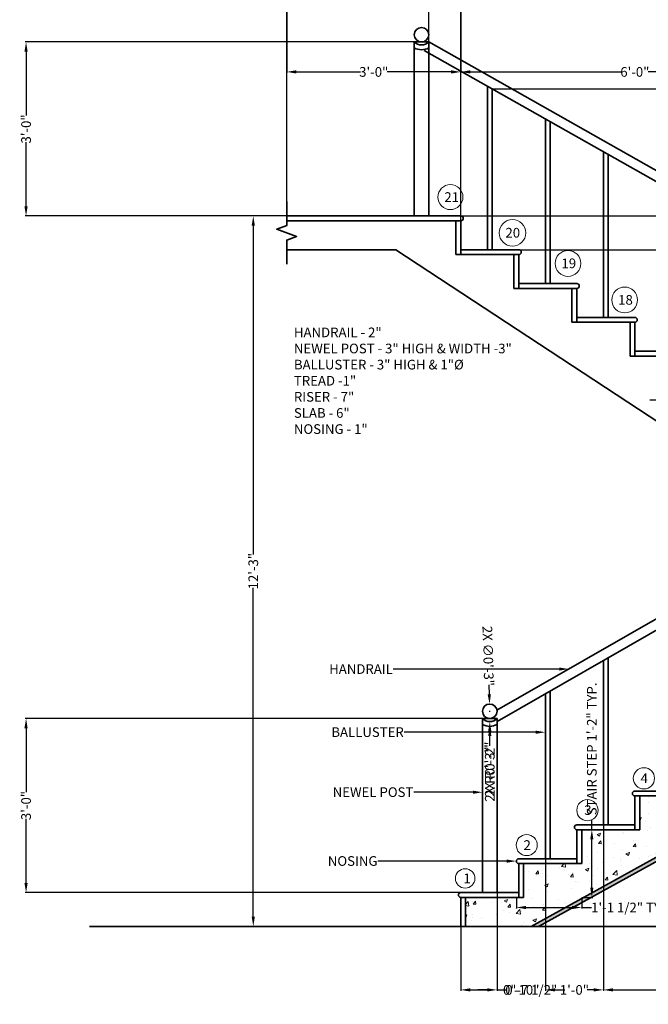
# Model space of a CAD drawing. Units: inches. Extents: x 865 to 1137, y 672 to 989.
# Tile 1 of 3: x 865 to 995, y 672 to 876. Entities that reach past the tile are written whole.
import ezdxf
from ezdxf import colors
from ezdxf.entities.mleader import LeaderData, LeaderLine
from ezdxf.math import Vec2, Vec3

# ---------------------------------------------------------------- set-up
doc = ezdxf.new("R2010")
doc.units = ezdxf.units.IN
doc.header["$LTSCALE"] = 0.1
doc.header["$MEASUREMENT"] = 0
for name, color, linetype, lineweight in [('A-ANNO-DIMS', 2, 'Continuous', 18), ('A-ANNO-SYMB', 3, 'Continuous', 18), ('A-ANNO-TEXT', 3, 'Continuous', 18), ('A-SECT', 7, 'Continuous', 35), ('A-SECT-PATT', 8, 'Continuous', 13)]:
    doc.layers.add(name, color=color, linetype=linetype, lineweight=lineweight)
doc.styles.get("Standard").update_dxf_attribs({"font": 'arial.ttf', "height": 2})
doc.dimstyles.get("Standard").update_dxf_attribs({"dimtxt": 2, "dimasz": 2, "dimexe": 0.18, "dimexo": 0.0625, "dimgap": 0.09, "dimtad": 0, "dimdec": 0, "dimzin": 0, "dimdsep": 46, "dimlunit": 3, "dimtxsty": 'Standard', "dimcen": 0.09, "dimadec": 0, "dimazin": 0, "dimtfac": 1, "dimtdec": 0, "dimtofl": 0, "dimtmove": 0, "dimatfit": 3, "dimfxl": 1, "dimtolj": 1, "dimtzin": 0, "dimarcsym": 0})

# ---------------------------------------------------------------- blocks, each defined once
blk = doc.blocks.new('*D6')
at = {"layer": 'A-ANNO-DIMS', "color": 0, "lineweight": -2, "transparency": 16777216}
for p, q in [((920.3, 835.55), (913.27, 835.55)), ((913.45, 833.55), (913.45, 765.48)), ((913.45, 690.55), (913.45, 758.62)), ((920.3, 688.55), (913.27, 688.55))]:
    blk.add_line(p, q, dxfattribs=at)
at = {"layer": 'A-ANNO-DIMS', "color": 0, "transparency": 16777216}
for points in [[(913.11, 833.55), (913.78, 833.55), (913.45, 835.55)], [(913.11, 690.55), (913.78, 690.55), (913.45, 688.55)]]:
    blk.add_solid(points, dxfattribs=at)
at = {"layer": 'Defpoints', "color": 0, "transparency": 16777216}
for p in [(920.36, 835.55), (913.45, 688.55), (920.36, 688.55)]:
    blk.add_point(p, dxfattribs=at)
at = {"layer": 'A-ANNO-DIMS', "color": 0, "transparency": 16777216, "insert": (913.45, 762.05), "char_height": 2, "attachment_point": 5, "rotation": 90}
blk.add_mtext('\\A1;12\'-3"', dxfattribs=at)
blk = doc.blocks.new('STAIR-STEP-SECT')
for p, q in [((13.5, 7), (13.5, 14)), ((0.5, 8), (12.5, 8)), ((0.5, 0), (0.5, 7)), ((0.5, 7), (13.5, 7))]:
    blk.add_line(p, q)
blk.add_arc((0.5, 7.5), 0.5, 90, 270)
blk = doc.blocks.new('*D9')
at = {"layer": 'A-ANNO-DIMS', "color": 0, "lineweight": -2, "transparency": 16777216}
for p, q in [((983.46, 708.55), (983.46, 710.55)), ((981.42, 708.55), (983.64, 708.55)), ((983.46, 696.55), (983.46, 706.55)), ((981.42, 694.55), (983.64, 694.55))]:
    blk.add_line(p, q, dxfattribs=at)
at = {"layer": 'A-ANNO-DIMS', "color": 0, "transparency": 16777216}
for points in [[(983.13, 706.55), (983.79, 706.55), (983.46, 708.55)], [(983.13, 696.55), (983.79, 696.55), (983.46, 694.55)]]:
    blk.add_solid(points, dxfattribs=at)
at = {"layer": 'Defpoints', "color": 0, "transparency": 16777216}
for p in [(981.36, 708.55), (983.46, 708.55), (981.36, 694.55)]:
    blk.add_point(p, dxfattribs=at)
at = {"layer": 'A-ANNO-DIMS', "color": 0, "transparency": 16777216, "insert": (983.46, 725.27), "char_height": 2, "attachment_point": 5, "rotation": 90}
blk.add_mtext('\\A1;STAIR STEP 1\'-2" TYP.', dxfattribs=at)
blk = doc.blocks.new('*D10')
at = {"layer": 'A-ANNO-DIMS', "color": 0, "lineweight": -2, "transparency": 16777216}
for p, q in [((967.86, 694.49), (967.86, 692.27)), ((981.36, 694.49), (981.36, 692.27)), ((969.86, 692.45), (979.36, 692.45)), ((981.36, 692.45), (983.36, 692.45))]:
    blk.add_line(p, q, dxfattribs=at)
at = {"layer": 'A-ANNO-DIMS', "color": 0, "transparency": 16777216}
for points in [[(969.86, 692.79), (969.86, 692.12), (967.86, 692.45)], [(979.36, 692.79), (979.36, 692.12), (981.36, 692.45)]]:
    blk.add_solid(points, dxfattribs=at)
at = {"layer": 'Defpoints', "color": 0, "transparency": 16777216}
for p in [(967.86, 694.55), (981.36, 694.55), (981.36, 692.45)]:
    blk.add_point(p, dxfattribs=at)
at = {"layer": 'A-ANNO-DIMS', "color": 0, "transparency": 16777216, "insert": (991.78, 692.45), "char_height": 2, "attachment_point": 5}
blk.add_mtext('\\A1;1\'-1 1/2" TYP.', dxfattribs=at)
blk = doc.blocks.new('*D12')
at = {"layer": 'A-ANNO-DIMS', "color": 0, "lineweight": -2, "transparency": 16777216}
for p, q in [((956.36, 891.19), (956.36, 865.17)), ((920.36, 880.69), (920.36, 865.17)), ((922.36, 865.35), (935.61, 865.35)), ((954.36, 865.35), (941.11, 865.35))]:
    blk.add_line(p, q, dxfattribs=at)
at = {"layer": 'A-ANNO-DIMS', "color": 0, "transparency": 16777216}
for points in [[(922.36, 865.69), (922.36, 865.02), (920.36, 865.35)], [(954.36, 865.69), (954.36, 865.02), (956.36, 865.35)]]:
    blk.add_solid(points, dxfattribs=at)
at = {"layer": 'Defpoints', "color": 0, "transparency": 16777216}
for p in [(956.36, 891.25), (920.36, 880.75), (956.36, 865.35)]:
    blk.add_point(p, dxfattribs=at)
at = {"layer": 'A-ANNO-DIMS', "color": 0, "transparency": 16777216, "insert": (938.36, 865.35), "char_height": 2, "attachment_point": 5}
blk.add_mtext('\\A1;3\'-0"', dxfattribs=at)
blk = doc.blocks.new('*D13')
at = {"layer": 'A-ANNO-DIMS', "color": 0, "lineweight": -2, "transparency": 16777216}
for p, q in [((956.36, 891.19), (956.36, 865.17)), ((1028.36, 880.69), (1028.36, 865.17)), ((958.36, 865.35), (989.6, 865.35)), ((1026.36, 865.35), (995.11, 865.35))]:
    blk.add_line(p, q, dxfattribs=at)
at = {"layer": 'A-ANNO-DIMS', "color": 0, "transparency": 16777216}
for points in [[(958.36, 865.69), (958.36, 865.02), (956.36, 865.35)], [(1026.36, 865.69), (1026.36, 865.02), (1028.36, 865.35)]]:
    blk.add_solid(points, dxfattribs=at)
at = {"layer": 'Defpoints', "color": 0, "transparency": 16777216}
for p in [(956.36, 891.25), (1028.36, 880.75), (1028.36, 865.35)]:
    blk.add_point(p, dxfattribs=at)
at = {"layer": 'A-ANNO-DIMS', "color": 0, "transparency": 16777216, "insert": (992.36, 865.35), "char_height": 2, "attachment_point": 5}
blk.add_mtext('\\A1;6\'-0"', dxfattribs=at)
blk = doc.blocks.new('*D21')
at = {"layer": 'A-ANNO-DIMS', "color": 0, "lineweight": -2, "transparency": 16777216}
for p, q in [((920.36, 835.61), (920.36, 887.89)), ((922.36, 887.71), (994.85, 887.71)), ((1078.86, 887.71), (1006.37, 887.71)), ((1080.86, 861.4), (1080.86, 887.89))]:
    blk.add_line(p, q, dxfattribs=at)
at = {"layer": 'A-ANNO-DIMS', "color": 0, "transparency": 16777216}
for points in [[(922.36, 888.04), (922.36, 887.37), (920.36, 887.71)], [(1078.86, 888.04), (1078.86, 887.37), (1080.86, 887.71)]]:
    blk.add_solid(points, dxfattribs=at)
at = {"layer": 'Defpoints', "color": 0, "transparency": 16777216}
for p in [(1080.86, 887.71), (1080.86, 861.34), (920.36, 835.55)]:
    blk.add_point(p, dxfattribs=at)
at = {"layer": 'A-ANNO-DIMS', "color": 0, "transparency": 16777216, "insert": (1000.61, 887.71), "char_height": 2, "attachment_point": 5}
blk.add_mtext('\\A1;13\'-4 1/2"', dxfattribs=at)
blk = doc.blocks.new('*D22')
at = {"layer": 'A-ANNO-DIMS', "color": 0, "lineweight": -2, "transparency": 16777216}
for p, q in [((985.86, 709.49), (985.86, 675.22)), ((1070.36, 688.49), (1070.36, 675.22)), ((987.86, 675.4), (1023.04, 675.4)), ((1068.36, 675.4), (1033.18, 675.4))]:
    blk.add_line(p, q, dxfattribs=at)
at = {"layer": 'A-ANNO-DIMS', "color": 0, "transparency": 16777216}
for points in [[(987.86, 675.74), (987.86, 675.07), (985.86, 675.4)], [(1068.36, 675.74), (1068.36, 675.07), (1070.36, 675.4)]]:
    blk.add_solid(points, dxfattribs=at)
at = {"layer": 'Defpoints', "color": 0, "transparency": 16777216}
for p in [(985.86, 709.55), (1070.36, 688.55), (1070.36, 675.4)]:
    blk.add_point(p, dxfattribs=at)
at = {"layer": 'A-ANNO-DIMS', "color": 0, "transparency": 16777216, "insert": (1028.11, 675.4), "char_height": 2, "attachment_point": 5}
blk.add_mtext('\\A1;7\'-0 1/2"', dxfattribs=at)
blk = doc.blocks.new('*D23')
at = {"layer": 'A-ANNO-DIMS', "color": 0, "lineweight": -2, "transparency": 16777216}
for p, q in [((960.8, 731.55), (866.28, 731.55)), ((866.46, 729.55), (866.46, 716.3)), ((866.46, 697.55), (866.46, 710.8)), ((960.8, 695.55), (866.28, 695.55))]:
    blk.add_line(p, q, dxfattribs=at)
at = {"layer": 'A-ANNO-DIMS', "color": 0, "transparency": 16777216}
for points in [[(866.12, 729.55), (866.79, 729.55), (866.46, 731.55)], [(866.12, 697.55), (866.79, 697.55), (866.46, 695.55)]]:
    blk.add_solid(points, dxfattribs=at)
at = {"layer": 'Defpoints', "color": 0, "transparency": 16777216}
for p in [(866.46, 731.55), (960.86, 731.55), (960.86, 695.55)]:
    blk.add_point(p, dxfattribs=at)
at = {"layer": 'A-ANNO-DIMS', "color": 0, "transparency": 16777216, "insert": (866.46, 713.55), "char_height": 2, "attachment_point": 5, "rotation": 90}
blk.add_mtext('\\A1;3\'-0"', dxfattribs=at)
blk = doc.blocks.new('*D24')
at = {"layer": 'A-ANNO-DIMS', "color": 0, "lineweight": -2, "transparency": 16777216}
for p, q in [((963.86, 695.49), (963.86, 675.22)), ((956.36, 688.49), (956.36, 675.22)), ((958.36, 675.4), (961.86, 675.4)), ((963.86, 675.4), (965.86, 675.4))]:
    blk.add_line(p, q, dxfattribs=at)
at = {"layer": 'A-ANNO-DIMS', "color": 0, "transparency": 16777216}
for points in [[(958.36, 675.74), (958.36, 675.07), (956.36, 675.4)], [(961.86, 675.74), (961.86, 675.07), (963.86, 675.4)]]:
    blk.add_solid(points, dxfattribs=at)
at = {"layer": 'Defpoints', "color": 0, "transparency": 16777216}
for p in [(963.86, 695.55), (956.36, 688.55), (963.86, 675.4)]:
    blk.add_point(p, dxfattribs=at)
at = {"layer": 'A-ANNO-DIMS', "color": 0, "transparency": 16777216, "insert": (970.94, 675.4), "char_height": 2, "attachment_point": 5}
blk.add_mtext('\\A1;0\'-7 1/2"', dxfattribs=at)
blk = doc.blocks.new('*D25')
at = {"layer": 'A-ANNO-DIMS', "color": 0, "lineweight": -2, "transparency": 16777216}
for p, q in [((962.92, 861.84), (1124.29, 861.84)), ((1124.11, 859.84), (1124.11, 850.29)), ((1124.11, 830.55), (1124.11, 840.1)), ((962.92, 828.55), (1124.29, 828.55))]:
    blk.add_line(p, q, dxfattribs=at)
at = {"layer": 'A-ANNO-DIMS', "color": 0, "transparency": 16777216}
for points in [[(1123.78, 859.84), (1124.44, 859.84), (1124.11, 861.84)], [(1123.78, 830.55), (1124.44, 830.55), (1124.11, 828.55)]]:
    blk.add_solid(points, dxfattribs=at)
at = {"layer": 'Defpoints', "color": 0, "transparency": 16777216}
for p in [(962.86, 861.84), (1124.11, 861.84), (962.86, 828.55)]:
    blk.add_point(p, dxfattribs=at)
at = {"layer": 'A-ANNO-DIMS', "color": 0, "transparency": 16777216, "insert": (1124.11, 845.19), "char_height": 2, "attachment_point": 5, "rotation": 90}
blk.add_mtext('\\A1;2\'-9 1/2"', dxfattribs=at)
blk = doc.blocks.new('*D26')
at = {"layer": 'A-ANNO-DIMS', "color": 0, "lineweight": -2, "transparency": 16777216}
for p, q in [((973.86, 702.49), (973.86, 675.22)), ((963.86, 695.49), (963.86, 675.22)), ((961.86, 675.4), (959.86, 675.4)), ((975.86, 675.4), (977.86, 675.4))]:
    blk.add_line(p, q, dxfattribs=at)
at = {"layer": 'A-ANNO-DIMS', "color": 0, "transparency": 16777216}
for points in [[(961.86, 675.74), (961.86, 675.07), (963.86, 675.4)], [(975.86, 675.74), (975.86, 675.07), (973.86, 675.4)]]:
    blk.add_solid(points, dxfattribs=at)
at = {"layer": 'Defpoints', "color": 0, "transparency": 16777216}
for p in [(973.86, 702.55), (963.86, 695.55), (973.86, 675.4)]:
    blk.add_point(p, dxfattribs=at)
at = {"layer": 'A-ANNO-DIMS', "color": 0, "transparency": 16777216, "insert": (968.86, 675.4), "char_height": 2, "attachment_point": 5}
blk.add_mtext('\\A1;0\'-10"', dxfattribs=at)
blk = doc.blocks.new('*D27')
at = {"layer": 'A-ANNO-DIMS', "color": 0, "lineweight": -2, "transparency": 16777216}
for p, q in [((985.86, 709.49), (985.86, 675.22)), ((973.86, 702.49), (973.86, 675.22)), ((975.86, 675.4), (977.2, 675.4)), ((983.86, 675.4), (982.51, 675.4))]:
    blk.add_line(p, q, dxfattribs=at)
at = {"layer": 'A-ANNO-DIMS', "color": 0, "transparency": 16777216}
for points in [[(975.86, 675.74), (975.86, 675.07), (973.86, 675.4)], [(983.86, 675.74), (983.86, 675.07), (985.86, 675.4)]]:
    blk.add_solid(points, dxfattribs=at)
at = {"layer": 'Defpoints', "color": 0, "transparency": 16777216}
for p in [(985.86, 709.55), (973.86, 702.55), (985.86, 675.4)]:
    blk.add_point(p, dxfattribs=at)
at = {"layer": 'A-ANNO-DIMS', "color": 0, "transparency": 16777216, "insert": (979.86, 675.4), "char_height": 2, "attachment_point": 5}
blk.add_mtext('\\A1;1\'-0"', dxfattribs=at)
blk = doc.blocks.new('*D28')
at = {"layer": 'A-ANNO-DIMS', "color": 0, "lineweight": -2, "transparency": 16777216}
for p, q in [((946.68, 871.55), (866.28, 871.55)), ((866.46, 869.55), (866.46, 856.3)), ((866.46, 837.55), (866.46, 850.8)), ((946.68, 835.55), (866.28, 835.55))]:
    blk.add_line(p, q, dxfattribs=at)
at = {"layer": 'A-ANNO-DIMS', "color": 0, "transparency": 16777216}
for points in [[(866.12, 869.55), (866.79, 869.55), (866.46, 871.55)], [(866.12, 837.55), (866.79, 837.55), (866.46, 835.55)]]:
    blk.add_solid(points, dxfattribs=at)
at = {"layer": 'Defpoints', "color": 0, "transparency": 16777216}
for p in [(866.46, 871.55), (946.74, 871.55), (946.74, 835.55)]:
    blk.add_point(p, dxfattribs=at)
at = {"layer": 'A-ANNO-DIMS', "color": 0, "transparency": 16777216, "insert": (866.46, 853.55), "char_height": 2, "attachment_point": 5, "rotation": 90}
blk.add_mtext('\\A1;3\'-0"', dxfattribs=at)
blk = doc.blocks.new('*D29')
at = {"layer": 'A-ANNO-DIMS', "color": 0, "lineweight": -2, "transparency": 16777216}
for p, q in [((949.74, 835.61), (949.74, 887.89)), ((951.74, 887.71), (954.36, 887.71)), ((956.36, 834.61), (956.36, 887.89)), ((956.36, 887.71), (958.36, 887.71))]:
    blk.add_line(p, q, dxfattribs=at)
at = {"layer": 'A-ANNO-DIMS', "color": 0, "transparency": 16777216}
for points in [[(951.74, 888.04), (951.74, 887.37), (949.74, 887.71)], [(954.36, 888.04), (954.36, 887.37), (956.36, 887.71)]]:
    blk.add_solid(points, dxfattribs=at)
at = {"layer": 'Defpoints', "color": 0, "transparency": 16777216}
for p in [(956.36, 887.71), (949.74, 835.55), (956.36, 834.55)]:
    blk.add_point(p, dxfattribs=at)
at = {"layer": 'A-ANNO-DIMS', "color": 0, "transparency": 16777216, "insert": (963.44, 887.71), "char_height": 2, "attachment_point": 5}
blk.add_mtext('\\A1;0\'-6 1/2"', dxfattribs=at)
blk = doc.blocks.new('*D31')
at = {"layer": 'A-ANNO-DIMS', "color": 0, "lineweight": -2, "transparency": 16777216}
for p, q in [((946.81, 835.55), (1124.29, 835.55)), ((1124.11, 833.55), (1124.11, 819.27)), ((1124.11, 799.49), (1124.11, 813.77)), ((995.46, 797.49), (1124.29, 797.49))]:
    blk.add_line(p, q, dxfattribs=at)
at = {"layer": 'A-ANNO-DIMS', "color": 0, "transparency": 16777216}
for points in [[(1123.78, 833.55), (1124.44, 833.55), (1124.11, 835.55)], [(1123.78, 799.49), (1124.44, 799.49), (1124.11, 797.49)]]:
    blk.add_solid(points, dxfattribs=at)
at = {"layer": 'Defpoints', "color": 0, "transparency": 16777216}
for p in [(946.74, 835.55), (1124.11, 835.55), (995.4, 797.49)]:
    blk.add_point(p, dxfattribs=at)
at = {"layer": 'A-ANNO-DIMS', "color": 0, "transparency": 16777216, "insert": (1124.11, 816.52), "char_height": 2, "attachment_point": 5, "rotation": 90}
blk.add_mtext('\\A1;3\'-2"', dxfattribs=at)
blk = doc.blocks.new('*D41')
at = {"layer": 'A-ANNO-DIMS', "color": 0, "lineweight": -2, "transparency": 16777216}
for p, q in [((962.19, 738.55), (962.25, 736.55)), ((962.27, 733.05), (962.45, 733.05)), ((962.36, 732.96), (962.36, 733.14))]:
    blk.add_line(p, q, dxfattribs=at)
at = {"layer": 'A-ANNO-DIMS', "color": 0, "transparency": 16777216}
blk.add_solid([(962.59, 736.56), (961.92, 736.54), (962.31, 734.56)], dxfattribs=at)
at = {"layer": 'Defpoints', "color": 0, "transparency": 16777216}
for p in [(962.31, 734.56), (962.4, 731.55)]:
    blk.add_point(p, dxfattribs=at)
at = {"layer": 'A-ANNO-DIMS', "color": 0, "transparency": 16777216, "insert": (962.02, 744.5), "char_height": 2, "attachment_point": 5, "rotation": 271.7169}
blk.add_mtext('\\A1;2X ∅0\'-3"', dxfattribs=at)
blk = doc.blocks.new('*D44')
at = {"layer": 'A-ANNO-DIMS', "color": 0, "lineweight": -2, "transparency": 16777216}
for p, q in [((962.27, 733.05), (962.45, 733.05)), ((962.36, 732.96), (962.36, 733.14)), ((962.36, 725.93), (962.36, 727.93))]:
    blk.add_line(p, q, dxfattribs=at)
at = {"layer": 'A-ANNO-DIMS', "color": 0, "transparency": 16777216}
blk.add_solid([(962.02, 727.93), (962.69, 727.93), (962.36, 729.93)], dxfattribs=at)
at = {"layer": 'Defpoints', "color": 0, "transparency": 16777216}
for p in [(962.36, 733.05), (962.36, 729.93)]:
    blk.add_point(p, dxfattribs=at)
at = {"layer": 'A-ANNO-DIMS', "color": 0, "transparency": 16777216, "insert": (962.36, 720.06), "char_height": 2, "attachment_point": 5, "rotation": 89.9939}
blk.add_mtext('\\A1;2X R0\'-3"', dxfattribs=at)
blk = doc.blocks.new('*D45')
at = {"layer": 'A-ANNO-DIMS', "color": 0, "lineweight": -2, "transparency": 16777216}
for p, q in [((962.27, 733.05), (962.45, 733.05)), ((962.36, 732.96), (962.36, 733.14)), ((962.36, 726.93), (962.36, 728.93))]:
    blk.add_line(p, q, dxfattribs=at)
at = {"layer": 'A-ANNO-DIMS', "color": 0, "transparency": 16777216}
blk.add_solid([(962.02, 728.93), (962.69, 728.93), (962.36, 730.93)], dxfattribs=at)
at = {"layer": 'Defpoints', "color": 0, "transparency": 16777216}
for p in [(962.36, 733.05), (962.36, 730.93)]:
    blk.add_point(p, dxfattribs=at)
at = {"layer": 'A-ANNO-DIMS', "color": 0, "transparency": 16777216, "insert": (962.36, 721.06), "char_height": 2, "attachment_point": 5, "rotation": 89.991}
blk.add_mtext('\\A1;2X R0\'-2"', dxfattribs=at)

msp = doc.modelspace()

# ---------------------------------------------------------------- hatches: boundary and pattern name
at = {"layer": 'A-SECT-PATT'}
h = msp.add_hatch(dxfattribs=at)
h.set_pattern_fill('AR-CONC', color=256)
h.set_pattern_definition([(50, (0, 0), (7.172602, -0.627521), [0.75, -8.25]), (355, (0, 0), (-1.387513, 7.52192), [0.6, -6.6]), (100.45144, (0.598, -0.052), (5.78509, 6.8944), [0.6374, -7.01142]), (46.1842, (0, 2), (10.672413, -1.65519), [1.125, -12.375]), (96.6356, (0.889, 1.862), (9.34662, 9.74119), [0.9561, -10.51714]), (351.1842, (0, 2), (9.34662, 9.74119), [0.9, -9.9]), (21, (1, 1.5), (5.96907, -4.02619), [0.75, -8.25]), (326, (1, 1.5), (2.433153, 7.2515), [0.6, -6.6]), (71.45144, (1.4974, 1.1645), (8.402224, 3.22531), [0.6374, -7.01142]), (37.5, (0, 0), (0.1215986, 3.3289385), [0, -6.52, 0, -6.7, 0, -6.625]), (7.5, (0, 0), (2.630695, 3.944117), [0, -3.82, 0, -6.37, 0, -2.525]), (327.5, (-2.23, 0), (5.3382244, -0.2255487), [0, -2.5, 0, -7.8, 0, -10.35]), (317.5, (-3.23, 0), (5.831862, 1.00105), [0, -3.25, 0, -5.18, 0, -7.35])])
h.paths.add_polyline_path([(1070.36, 743.46), (1077.35, 743.46), (1077.35, 750.55), (1059.06, 750.55), (1059.06, 743.55), (1045.43, 743.55), (1045.43, 736.55), (1029.36, 736.55), (1029.36, 729.55), (1017.36, 729.55), (1017.36, 722.55), (1005.36, 722.55), (1005.36, 715.55), (993.36, 715.55), (993.36, 708.55), (981.36, 708.55), (981.36, 701.55), (969.36, 701.55), (969.36, 694.55), (957.36, 694.55), (957.36, 688.55), (970.9, 688.55)])
h = msp.add_hatch(dxfattribs=at)
h.set_pattern_fill('AR-CONC', color=256, scale=0.4)
h.set_pattern_definition([(50, (0, 0), (2.8690407, -0.2510085), [0.3, -3.3]), (355, (0, 0), (-0.5550053, 3.0087685), [0.24, -2.64]), (100.45144, (0.239, -0.021), (2.3140354, 2.75776), [0.254961, -2.8045684]), (46.1842, (0, 0.8), (4.268965, -0.662077), [0.45, -4.95]), (96.63564, (0.3557, 0.745), (3.738648, 3.896474), [0.382441, -4.206855]), (351.18416, (0, 0.8), (3.738648, 3.896474), [0.36, -3.96]), (21, (0.4, 0.6), (2.387628, -1.6104756), [0.3, -3.3]), (326, (0.4, 0.6), (0.973261, 2.9006), [0.24, -2.64]), (71.45144, (0.599, 0.4658), (3.3608895, 1.2901246), [0.254961, -2.8045684]), (37.5, (0, 0), (0.0486394, 1.3315754), [0, -2.608, 0, -2.68, 0, -2.65]), (7.5, (0, 0), (1.0522781, 1.5776468), [0, -1.528, 0, -2.548, 0, -1.01]), (327.5, (-0.892, 0), (2.13528974, -0.0902195), [0, -1, 0, -3.12, 0, -4.14]), (317.5, (-1.292, 0), (2.3327447, 0.40042), [0, -1.3, 0, -2.072, 0, -2.94])])
h.paths.add_polyline_path([(1070.36, 742.6), (1070.36, 743.46), (970.9, 688.55), (972.46, 688.55)])

# ---------------------------------------------------------------- linework, layer by layer
at = {"layer": 'A-ANNO-SYMB'}
for centre, radius in [((954.22, 839.45), 2.59), ((967.05, 832.05), 2.75), ((978.53, 825.72), 2.67), ((990.25, 818.16), 2.67), ((994.23, 719.18), 2.2), ((982.55, 712.58), 2.19), ((970, 705.36), 2.18), ((957.27, 698.47), 2.01)]:
    msp.add_circle(centre, radius, dxfattribs=at)
at = {"layer": 'A-SECT'}
for p, q in [((949.74, 871.55), (946.74, 871.55)), ((946.74, 871.55), (946.74, 835.55)), ((949.74, 835.55), (949.74, 871.55)), ((949.74, 871.55), (1016.07, 834.04)), ((948.76, 869.81), (1015.09, 832.3)), ((961.86, 862.4), (961.86, 828.55)), ((962.86, 828.55), (962.86, 861.84)), ((973.86, 855.62), (973.86, 821.55)), ((974.86, 821.55), (974.86, 855.05)), ((985.86, 848.83), (985.86, 814.55)), ((986.86, 814.55), (986.86, 848.27)), ((956.36, 835.55), (920.36, 835.55)), ((956.36, 834.55), (920.36, 834.55)), ((956.36, 827.55), (956.36, 834.55)), ((942.92, 828.55), (920.36, 828.55)), ((942.92, 828.55), (1030.37, 771.05)), ((963.86, 730.97), (1022.85, 764.82)), ((963.85, 733.27), (1015.3, 762.79)), ((986.86, 709.55), (986.86, 744.16)), ((970.9, 688.55), (1070.36, 743.46)), ((972.46, 688.55), (1070.72, 742.8)), ((985.86, 743.59), (985.86, 709.55)), ((973.86, 736.7), (973.86, 702.55)), ((974.86, 702.55), (974.86, 737.28)), ((963.86, 731.55), (960.86, 731.55)), ((960.86, 731.55), (960.86, 695.55)), ((963.86, 695.55), (963.86, 731.55)), ((969.36, 694.55), (969.36, 701.55)), ((956.36, 695.55), (968.36, 695.55)), ((956.36, 688.55), (956.36, 694.55)), ((956.36, 694.55), (969.36, 694.55)), ((957.36, 688.55), (957.36, 694.55)), ((1110.96, 688.55), (879.61, 688.55))]:
    msp.add_line(p, q, dxfattribs=at)
msp.add_lwpolyline([(920.36, 838.55), (920.36, 833.55), (918.3, 832.8), (922.42, 831.3), (920.36, 830.55), (920.36, 825.55)], dxfattribs=at)
for centre in [(948.24, 873.05), (962.36, 733.05)]:
    msp.add_circle(centre, 1.5, dxfattribs=at)
for centre, radius, start, end in [((948.24, 873.05), 2.12, 224.9939, 315.0061), ((948.24, 873.05), 3.12, 241.2754, 298.7246), ((956.36, 835.05), 0.5, 270, 450), ((962.36, 733.05), 2.12, 224.9939, 315.0061), ((962.36, 733.05), 3.12, 241.2754, 298.7246), ((956.36, 695.05), 0.5, 90, 270)]:
    msp.add_arc(centre, radius, start, end, dxfattribs=at)

# ---------------------------------------------------------------- block references
at = {"layer": 'A-SECT', "extrusion": (0, 0, -1), "zscale": -1}
for p in [(-968.86, 820.55), (-980.86, 813.55), (-992.86, 806.55), (-1004.86, 799.55)]:
    msp.add_blockref('STAIR-STEP-SECT', p, dxfattribs=at)
at = {"layer": 'A-SECT'}
for p in [(991.86, 708.55), (979.86, 701.55), (967.86, 694.55)]:
    msp.add_blockref('STAIR-STEP-SECT', p, dxfattribs=at)

# ---------------------------------------------------------------- texts
at = {"layer": 'A-ANNO-TEXT', "char_height": 2, "attachment_point": 1}
for s, width, insert in [('21', 1.0762, (952.96, 840.45)), ('20', 1.0762, (965.6, 833.07)), ('19', 1.0762, (977.19, 826.74)), ('18', 1.0762, (988.91, 819.18)), ('HANDRAIL - 2"\\PNEWEL POST - 3" HIGH & WIDTH -3"\\PBALLUSTER - 3" HIGH & 1"%%C\\PTREAD -1"\\PRISER - 7"\\PSLAB - 6"\\PNOSING - 1"', 50.113, (921.85, 812.45)), ('4', 1.0762, (993.54, 720.18)), ('3', 1.0762, (981.9, 713.6)), ('2', 1.0762, (969.34, 706.37)), ('1', 1.0762, (956.9, 699.47))]:
    msp.add_mtext_dynamic_manual_height_columns(s, width=width, gutter_width=10, heights=[0], dxfattribs=dict(at, insert=insert))

# ---------------------------------------------------------------- dimensions: what is measured, and where the dimension line sits
at = {"layer": 'A-ANNO-DIMS'}
for base, p1, p2, picture, middle in [((956.36, 865.35), (920.36, 880.75), (956.36, 891.25), '*D12', (938.36, 865.35)), ((1080.86, 887.71), (920.36, 835.55), (1080.86, 861.34), '*D21', (1000.61, 887.71)), ((956.36, 887.71), (949.74, 835.55), (956.36, 834.55), '*D29', (963.44, 887.71)), ((1028.36, 865.35), (956.36, 891.25), (1028.36, 880.75), '*D13', (992.36, 865.35)), ((985.86, 675.4), (973.86, 702.55), (985.86, 709.55), '*D27', (979.86, 675.4)), ((1070.36, 675.4), (985.86, 709.55), (1070.36, 688.55), '*D22', (1028.11, 675.4)), ((973.86, 675.4), (963.86, 695.55), (973.86, 702.55), '*D26', (968.86, 675.4)), ((963.86, 675.4), (956.36, 688.55), (963.86, 695.55), '*D24', (970.94, 675.4))]:
    dim = msp.add_linear_dim(base=base, p1=p1, p2=p2, dimstyle='Standard', override={"dimdec": 1, "dimlfac": 1, "dimrnd": 0, "dimzin": 1, "dimdsep": 46, "dimlunit": 4, "dimfrac": 2}, dxfattribs=at)
    dim.commit()
    dim.dimension.update_dxf_attribs({"geometry": picture, "text_midpoint": middle})
for base, p1, p2, override, picture, middle in [((866.46, 871.55), (946.74, 835.55), (946.74, 871.55), {"dimdec": 1, "dimlfac": 1, "dimrnd": 0, "dimzin": 1, "dimdsep": 46, "dimlunit": 4, "dimfrac": 2}, '*D28', (866.46, 853.55)), ((1124.11, 861.84), (962.86, 828.55), (962.86, 861.84), {"dimdec": 1, "dimlfac": 1, "dimrnd": 0, "dimzin": 1, "dimdsep": 46, "dimlunit": 4, "dimfrac": 2}, '*D25', (1124.11, 845.19)), ((913.45, 688.55), (920.36, 835.55), (920.36, 688.55), {"dimclrd": 0, "dimclre": 0, "dimclrt": 0}, '*D6', (913.45, 762.05)), ((1124.11, 835.55), (995.4, 797.49), (946.74, 835.55), {"dimdec": 1, "dimlfac": 1, "dimrnd": 0, "dimzin": 1, "dimdsep": 46, "dimlunit": 4, "dimfrac": 2}, '*D31', (1124.11, 816.52)), ((866.46, 731.55), (960.86, 695.55), (960.86, 731.55), {"dimdec": 1, "dimlfac": 1, "dimrnd": 0, "dimzin": 1, "dimdsep": 46, "dimlunit": 4, "dimfrac": 2}, '*D23', (866.46, 713.55))]:
    dim = msp.add_linear_dim(base=base, p1=p1, p2=p2, angle=90, dimstyle='Standard', override=override, dxfattribs=at)
    dim.commit()
    dim.dimension.update_dxf_attribs({"geometry": picture, "text_midpoint": middle})
dim = msp.add_diameter_dim_2p(p1=(962.4, 731.55), p2=(962.31, 734.56), text='2X <>', dimstyle='Standard', override={"dimdec": 1, "dimlfac": 1, "dimrnd": 0, "dimzin": 1, "dimdsep": 46, "dimlunit": 4, "dimfrac": 2}, dxfattribs=at)
dim.commit()
dim.dimension.update_dxf_attribs({"geometry": '*D41', "text_midpoint": (962.02, 744.5), "dimtype": 163})
dim = msp.add_linear_dim(base=(983.46, 708.55), p1=(981.36, 694.55), p2=(981.36, 708.55), angle=90, text='STAIR STEP <> TYP.', dimstyle='Standard', override={"dimdec": 1, "dimrnd": 0, "dimzin": 1, "dimlunit": 4, "dimfrac": 2}, dxfattribs=at)
dim.commit()
dim.dimension.update_dxf_attribs({"geometry": '*D9', "text_midpoint": (983.46, 725.27)})
for mpoint, picture, middle in [((962.36, 729.93), '*D44', (962.36, 720.06)), ((962.36, 730.93), '*D45', (962.36, 721.06))]:
    dim = msp.add_radius_dim(center=(962.36, 733.05), mpoint=mpoint, text='2X <>', dimstyle='Standard', override={"dimdec": 1, "dimlfac": 1, "dimrnd": 0, "dimzin": 1, "dimdsep": 46, "dimlunit": 4, "dimfrac": 2}, dxfattribs=at)
    dim.commit()
    dim.dimension.update_dxf_attribs({"geometry": picture, "text_midpoint": middle})
dim = msp.add_linear_dim(base=(981.36, 692.45), p1=(967.86, 694.55), p2=(981.36, 694.55), text='<> TYP.', dimstyle='Standard', override={"dimdec": 1, "dimrnd": 0, "dimzin": 1, "dimlunit": 4, "dimfrac": 2}, dxfattribs=at)
dim.commit()
dim.dimension.update_dxf_attribs({"geometry": '*D10', "text_midpoint": (991.78, 692.45)})

# ---------------------------------------------------------------- leaders
at = {"layer": 'A-ANNO-TEXT'}
ml = msp.add_multileader_mtext('Standard', dxfattribs=at)
ml.set_content('HANDRAIL', color=256)
ml.set_leader_properties()
ml.build(insert=Vec2(0, 0))
ml.multileader.update_dxf_attribs({"dogleg_length": 0.36, "arrow_head_size": 2})
ctx = ml.context
ctx.base_point, ctx.char_height, ctx.arrow_head_size, ctx.landing_gap_size, ctx.plane_origin = Vec3(928.42, 741.79), 2, 2, 0.09, Vec3(978.71, 741.79)
ctx.text_align_type = 2
notes = []
notes.append((ctx, [(0, (1, 1, 0), (942.76, 741.79), (-1, 0), 0.36, [(0, [(978.71, 741.79)], 0, [])])]))
ctx.mtext.insert, ctx.mtext.alignment, ctx.mtext.flow_direction = Vec3(942.31, 742.79), 3, 5
ml = msp.add_multileader_mtext('Standard', dxfattribs=at)
ml.set_content('BALLUSTER', color=256)
ml.set_leader_properties()
ml.build(insert=Vec2(0, 0))
ml.multileader.update_dxf_attribs({"dogleg_length": 0.36, "arrow_head_size": 2})
ctx = ml.context
ctx.base_point, ctx.char_height, ctx.arrow_head_size, ctx.landing_gap_size, ctx.plane_origin = Vec3(928.42, 728.72), 2, 2, 0.09, Vec3(973.86, 728.72)
ctx.text_align_type = 2
notes.append((ctx, [(0, (1, 1, 0), (945.02, 728.72), (-1, 0), 0.36, [(0, [(973.86, 728.72)], 0, [])])]))
ctx.mtext.insert, ctx.mtext.alignment, ctx.mtext.flow_direction = Vec3(944.57, 729.74), 3, 5
ml = msp.add_multileader_mtext('Standard', dxfattribs=at)
ml.set_content('NEWEL POST', color=256)
ml.set_leader_properties()
ml.build(insert=Vec2(0, 0))
ml.multileader.update_dxf_attribs({"dogleg_length": 0.36, "arrow_head_size": 2})
ctx = ml.context
ctx.base_point, ctx.char_height, ctx.arrow_head_size, ctx.landing_gap_size, ctx.plane_origin = Vec3(928.42, 716.3), 2, 2, 0.09, Vec3(960.86, 716.3)
ctx.text_align_type = 2
notes.append((ctx, [(0, (1, 1, 0), (947.01, 716.3), (-1, 0), 0.36, [(0, [(960.86, 716.3)], 0, [])])]))
ctx.mtext.insert, ctx.mtext.alignment, ctx.mtext.flow_direction = Vec3(946.56, 717.32), 3, 5
ml = msp.add_multileader_mtext('Standard', dxfattribs=at)
ml.set_content('NOSING ', color=256)
ml.set_leader_properties()
ml.build(insert=Vec2(0, 0))
ml.multileader.update_dxf_attribs({"dogleg_length": 0.36, "arrow_head_size": 2})
ctx = ml.context
ctx.base_point, ctx.char_height, ctx.arrow_head_size, ctx.landing_gap_size, ctx.plane_origin = Vec3(928.42, 702.05), 2, 2, 0.09, Vec3(967.86, 702.05)
ctx.text_align_type = 2
notes.append((ctx, [(0, (1, 1, 0), (939.59, 702.05), (-1, 0), 0.36, [(0, [(967.86, 702.05)], 0, [])])]))
ctx.mtext.insert, ctx.mtext.alignment, ctx.mtext.flow_direction = Vec3(939.14, 703.07), 3, 5
for ctx, leaders in notes:
    for number, flags, end, landing, length, lines in leaders:
        leader = LeaderData()
        leader.index, (leader.has_last_leader_line, leader.has_dogleg_vector, leader.attachment_direction) = number, flags
        leader.last_leader_point, leader.dogleg_vector, leader.dogleg_length = Vec3(end), Vec3(landing), length
        for number, points, colour, breaks in lines:
            line = LeaderLine()
            line.index, line.vertices, line.color, line.breaks = number, Vec3.list(points), colors.encode_raw_color(colour), breaks
            leader.lines.append(line)
        ctx.leaders.append(leader)

doc.saveas('drawing.dxf')
